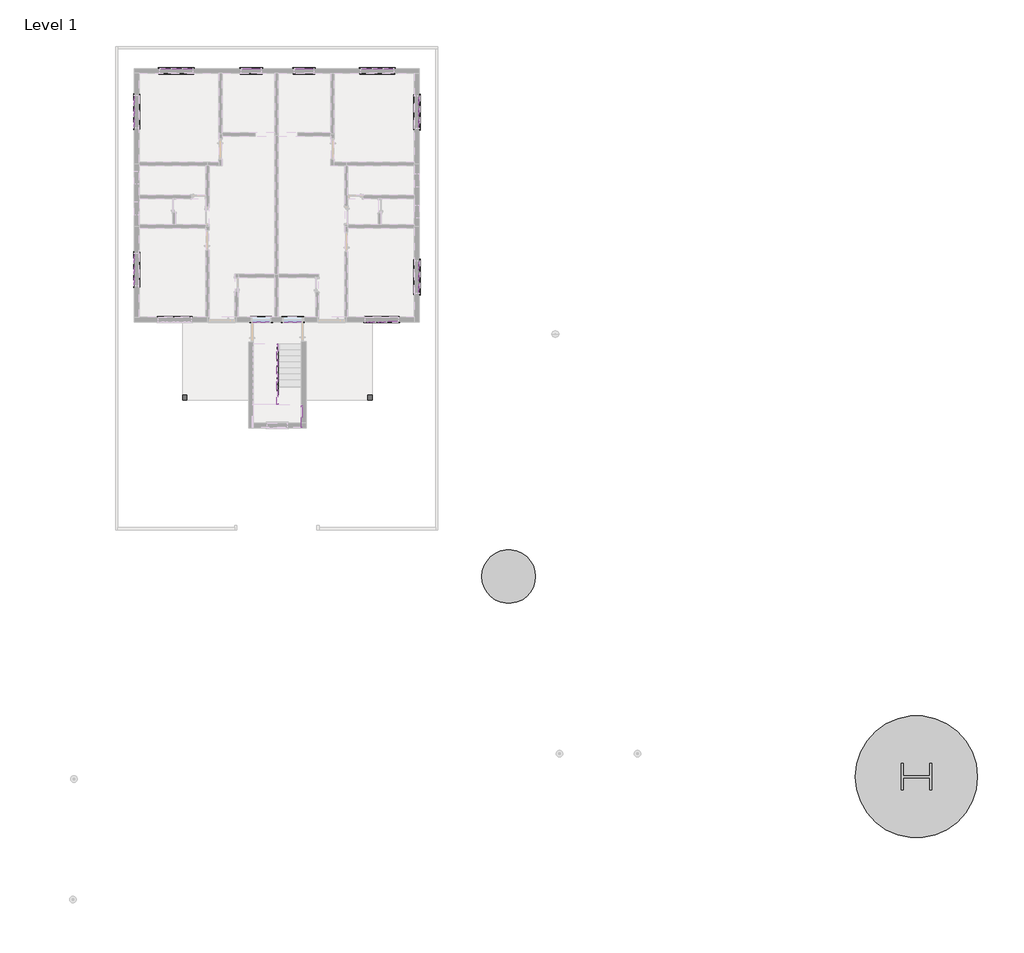
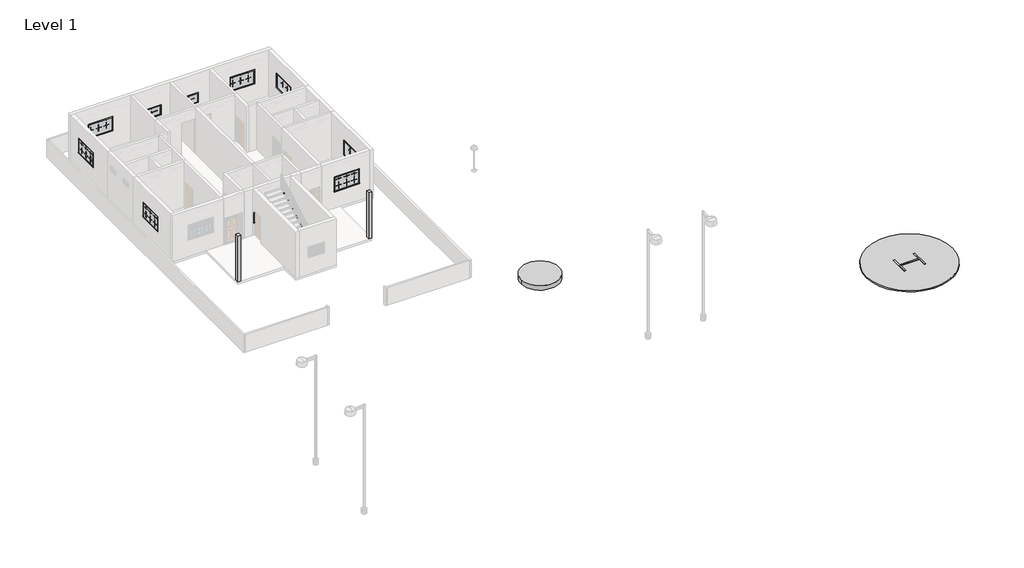
# One storey, part 4 of 4: 75 proxies, 5 members.
"""IFC4 building model written with IfcOpenShell, lengths in millimetres."""

from ifc_helpers import new_model, si_unit, frame, origin, place, context, project, spatial, polyline, outline, extrude, transform, mapped, element, save
from components import roads_7a27419f, generic_models_1_generic_models_1_f4687d58, m_muntin_pattern_2x2_m_muntin_pattern_2x2_be83c6ce, m_muntin_pattern_2x2_m_muntin_pattern_2x2_d2526705, m_muntin_pattern_2x2_m_muntin_pattern_2x2_b257745b, m_muntin_pattern_2x2_m_muntin_pattern_2x2_3c44882e, m_muntin_pattern_2x2_m_muntin_pattern_2x2_c118e93d, m_trim_window_exterior_flat_with_sill_30a8f3cc, m_trim_window_exterior_flat_with_sill_78b3ef69, m_trim_window_interior_flat_picture_frame_90bf1a90, m_trim_window_interior_flat_picture_frame_87bc748b

model = new_model("IFC4")

# Units and contexts
model_context = context("Model", 3, world=origin())
ifc_project = project(units=[si_unit("LENGTHUNIT", "METRE", prefix="MILLI")], contexts=[model_context])

# Site, building, storey
site = spatial("IfcSite", under=ifc_project)
building = spatial("IfcBuilding", under=site)
storey = spatial("IfcBuildingStorey", under=building, Name="Level 1", Elevation=0.0)

# Proxies
placement = place(None, origin())
roads_shape = roads_7a27419f(model_context)
element("IfcBuildingElementProxy", 1, Name="Roads", at=placement, inside=storey, context=model_context, shape_type="MappedRepresentation", body=[
    mapped(roads_shape, transform((0.0, 0.0, 0.0), x_axis=(1.0, 0.0, 0.0), y_axis=(0.0, 1.0, 0.0), z_axis=(0.0, 0.0, 1.0))),
])
generic_models_1_generic_models_1_shape = generic_models_1_generic_models_1_f4687d58(model_context)
element("IfcBuildingElementProxy", 2, Name="Generic Models 1 : Generic Models 1", ObjectType="Generic Models 1 : Generic Models 1", at=placement, inside=storey, context=model_context, shape_type="MappedRepresentation", body=[
    mapped(generic_models_1_generic_models_1_shape, transform((0.0, 0.0, 0.0), x_axis=(1.0, 0.0, 0.0), y_axis=(0.0, 1.0, 0.0), z_axis=(0.0, 0.0, 1.0))),
])
m_muntin_pattern_2x2_m_muntin_pattern_2x2_shape = m_muntin_pattern_2x2_m_muntin_pattern_2x2_be83c6ce(model_context)
element("IfcBuildingElementProxy", 3, Name="M_Muntin Pattern_2x2 : M_Muntin Pattern_2x2", ObjectType="M_Muntin Pattern_2x2 : M_Muntin Pattern_2x2", at=placement, inside=storey, context=model_context, shape_type="MappedRepresentation", body=[
    mapped(m_muntin_pattern_2x2_m_muntin_pattern_2x2_shape, transform((-12105.0132915, 19636.711641, 1289.05), x_axis=(1.0, 0.0, 0.0), y_axis=(0.0, 1.0, 0.0), z_axis=(0.0, 0.0, 1.0))),
])
element("IfcBuildingElementProxy", 4, Name="M_Muntin Pattern_2x2 : M_Muntin Pattern_2x2", ObjectType="M_Muntin Pattern_2x2 : M_Muntin Pattern_2x2", at=placement, inside=storey, context=model_context, shape_type="MappedRepresentation", body=[
    mapped(m_muntin_pattern_2x2_m_muntin_pattern_2x2_shape, transform((-13532.7049582, 17146.4533076, 1289.05), x_axis=(0.0, 1.0, 0.0), y_axis=(-1.0, 0.0, 0.0), z_axis=(0.0, 0.0, 1.0))),
])
element("IfcBuildingElementProxy", 5, Name="M_Muntin Pattern_2x2 : M_Muntin Pattern_2x2", ObjectType="M_Muntin Pattern_2x2 : M_Muntin Pattern_2x2", at=placement, inside=storey, context=model_context, shape_type="MappedRepresentation", body=[
    mapped(m_muntin_pattern_2x2_m_muntin_pattern_2x2_shape, transform((-2808.6132915, 19636.711641, 1289.05), x_axis=(1.0, 0.0, 0.0), y_axis=(0.0, 1.0, 0.0), z_axis=(0.0, 0.0, 1.0))),
])
element("IfcBuildingElementProxy", 6, Name="M_Muntin Pattern_2x2 : M_Muntin Pattern_2x2", ObjectType="M_Muntin Pattern_2x2 : M_Muntin Pattern_2x2", at=placement, inside=storey, context=model_context, shape_type="MappedRepresentation", body=[
    mapped(m_muntin_pattern_2x2_m_muntin_pattern_2x2_shape, transform((-369.1549582, 18132.8199743, 1289.05), x_axis=(0.0, -1.0, 0.0), y_axis=(1.0, 0.0, 0.0), z_axis=(0.0, 0.0, 1.0))),
])
element("IfcBuildingElementProxy", 7, Name="M_Muntin Pattern_2x2 : M_Muntin Pattern_2x2", ObjectType="M_Muntin Pattern_2x2 : M_Muntin Pattern_2x2", at=placement, inside=storey, context=model_context, shape_type="MappedRepresentation", body=[
    mapped(m_muntin_pattern_2x2_m_muntin_pattern_2x2_shape, transform((-369.1549582, 10487.4199743, 1289.05), x_axis=(0.0, -1.0, 0.0), y_axis=(1.0, 0.0, 0.0), z_axis=(0.0, 0.0, 1.0))),
])
element("IfcBuildingElementProxy", 8, Name="M_Muntin Pattern_2x2 : M_Muntin Pattern_2x2", ObjectType="M_Muntin Pattern_2x2 : M_Muntin Pattern_2x2", at=placement, inside=storey, context=model_context, shape_type="MappedRepresentation", body=[
    mapped(m_muntin_pattern_2x2_m_muntin_pattern_2x2_shape, transform((-1599.9966249, 7920.961641, 1289.05), x_axis=(-1.0, 0.0, 0.0), y_axis=(0.0, -1.0, 0.0), z_axis=(0.0, 0.0, 1.0))),
])
element("IfcBuildingElementProxy", 9, Name="M_Muntin Pattern_2x2 : M_Muntin Pattern_2x2", ObjectType="M_Muntin Pattern_2x2 : M_Muntin Pattern_2x2", at=placement, inside=storey, context=model_context, shape_type="MappedRepresentation", body=[
    mapped(m_muntin_pattern_2x2_m_muntin_pattern_2x2_shape, transform((-13532.7049582, 9834.4283076, 1289.05), x_axis=(0.0, 1.0, 0.0), y_axis=(-1.0, 0.0, 0.0), z_axis=(0.0, 0.0, 1.0))),
])
m_muntin_pattern_2x2_m_muntin_pattern_2x2_2_shape = m_muntin_pattern_2x2_m_muntin_pattern_2x2_d2526705(model_context)
element("IfcBuildingElementProxy", 10, Name="M_Muntin Pattern_2x2 : M_Muntin Pattern_2x2", ObjectType="M_Muntin Pattern_2x2 : M_Muntin Pattern_2x2", at=placement, inside=storey, context=model_context, shape_type="MappedRepresentation", body=[
    mapped(m_muntin_pattern_2x2_m_muntin_pattern_2x2_2_shape, transform((-11093.2466249, 19636.711641, 1289.05), x_axis=(-1.0, 0.0, 0.0), y_axis=(0.0, -1.0, 0.0), z_axis=(0.0, 0.0, 1.0))),
])
element("IfcBuildingElementProxy", 11, Name="M_Muntin Pattern_2x2 : M_Muntin Pattern_2x2", ObjectType="M_Muntin Pattern_2x2 : M_Muntin Pattern_2x2", at=placement, inside=storey, context=model_context, shape_type="MappedRepresentation", body=[
    mapped(m_muntin_pattern_2x2_m_muntin_pattern_2x2_2_shape, transform((-11599.1299582, 19636.711641, 1289.05), x_axis=(-1.0, 0.0, 0.0), y_axis=(0.0, -1.0, 0.0), z_axis=(0.0, 0.0, 1.0))),
])
element("IfcBuildingElementProxy", 12, Name="M_Muntin Pattern_2x2 : M_Muntin Pattern_2x2", ObjectType="M_Muntin Pattern_2x2 : M_Muntin Pattern_2x2", at=placement, inside=storey, context=model_context, shape_type="MappedRepresentation", body=[
    mapped(m_muntin_pattern_2x2_m_muntin_pattern_2x2_2_shape, transform((-13532.7049582, 18158.2199743, 1289.05), x_axis=(0.0, -1.0, 0.0), y_axis=(1.0, 0.0, 0.0), z_axis=(0.0, 0.0, 1.0))),
])
element("IfcBuildingElementProxy", 13, Name="M_Muntin Pattern_2x2 : M_Muntin Pattern_2x2", ObjectType="M_Muntin Pattern_2x2 : M_Muntin Pattern_2x2", at=placement, inside=storey, context=model_context, shape_type="MappedRepresentation", body=[
    mapped(m_muntin_pattern_2x2_m_muntin_pattern_2x2_2_shape, transform((-13532.7049582, 17652.336641, 1289.05), x_axis=(0.0, -1.0, 0.0), y_axis=(1.0, 0.0, 0.0), z_axis=(0.0, 0.0, 1.0))),
])
element("IfcBuildingElementProxy", 14, Name="M_Muntin Pattern_2x2 : M_Muntin Pattern_2x2", ObjectType="M_Muntin Pattern_2x2 : M_Muntin Pattern_2x2", at=placement, inside=storey, context=model_context, shape_type="MappedRepresentation", body=[
    mapped(m_muntin_pattern_2x2_m_muntin_pattern_2x2_2_shape, transform((-1796.8466249, 19636.711641, 1289.05), x_axis=(-1.0, 0.0, 0.0), y_axis=(0.0, -1.0, 0.0), z_axis=(0.0, 0.0, 1.0))),
])
element("IfcBuildingElementProxy", 15, Name="M_Muntin Pattern_2x2 : M_Muntin Pattern_2x2", ObjectType="M_Muntin Pattern_2x2 : M_Muntin Pattern_2x2", at=placement, inside=storey, context=model_context, shape_type="MappedRepresentation", body=[
    mapped(m_muntin_pattern_2x2_m_muntin_pattern_2x2_2_shape, transform((-2302.7299582, 19636.711641, 1289.05), x_axis=(-1.0, 0.0, 0.0), y_axis=(0.0, -1.0, 0.0), z_axis=(0.0, 0.0, 1.0))),
])
element("IfcBuildingElementProxy", 16, Name="M_Muntin Pattern_2x2 : M_Muntin Pattern_2x2", ObjectType="M_Muntin Pattern_2x2 : M_Muntin Pattern_2x2", at=placement, inside=storey, context=model_context, shape_type="MappedRepresentation", body=[
    mapped(m_muntin_pattern_2x2_m_muntin_pattern_2x2_2_shape, transform((-369.1549582, 17121.0533076, 1289.05), x_axis=(0.0, 1.0, 0.0), y_axis=(-1.0, 0.0, 0.0), z_axis=(0.0, 0.0, 1.0))),
])
element("IfcBuildingElementProxy", 17, Name="M_Muntin Pattern_2x2 : M_Muntin Pattern_2x2", ObjectType="M_Muntin Pattern_2x2 : M_Muntin Pattern_2x2", at=placement, inside=storey, context=model_context, shape_type="MappedRepresentation", body=[
    mapped(m_muntin_pattern_2x2_m_muntin_pattern_2x2_2_shape, transform((-369.1549582, 17626.936641, 1289.05), x_axis=(0.0, 1.0, 0.0), y_axis=(-1.0, 0.0, 0.0), z_axis=(0.0, 0.0, 1.0))),
])
element("IfcBuildingElementProxy", 18, Name="M_Muntin Pattern_2x2 : M_Muntin Pattern_2x2", ObjectType="M_Muntin Pattern_2x2 : M_Muntin Pattern_2x2", at=placement, inside=storey, context=model_context, shape_type="MappedRepresentation", body=[
    mapped(m_muntin_pattern_2x2_m_muntin_pattern_2x2_2_shape, transform((-369.1549582, 9475.6533076, 1289.05), x_axis=(0.0, 1.0, 0.0), y_axis=(-1.0, 0.0, 0.0), z_axis=(0.0, 0.0, 1.0))),
])
element("IfcBuildingElementProxy", 19, Name="M_Muntin Pattern_2x2 : M_Muntin Pattern_2x2", ObjectType="M_Muntin Pattern_2x2 : M_Muntin Pattern_2x2", at=placement, inside=storey, context=model_context, shape_type="MappedRepresentation", body=[
    mapped(m_muntin_pattern_2x2_m_muntin_pattern_2x2_2_shape, transform((-369.1549582, 9981.536641, 1289.05), x_axis=(0.0, 1.0, 0.0), y_axis=(-1.0, 0.0, 0.0), z_axis=(0.0, 0.0, 1.0))),
])
element("IfcBuildingElementProxy", 20, Name="M_Muntin Pattern_2x2 : M_Muntin Pattern_2x2", ObjectType="M_Muntin Pattern_2x2 : M_Muntin Pattern_2x2", at=placement, inside=storey, context=model_context, shape_type="MappedRepresentation", body=[
    mapped(m_muntin_pattern_2x2_m_muntin_pattern_2x2_2_shape, transform((-2611.7632915, 7920.961641, 1289.05), x_axis=(1.0, 0.0, 0.0), y_axis=(0.0, 1.0, 0.0), z_axis=(0.0, 0.0, 1.0))),
])
element("IfcBuildingElementProxy", 21, Name="M_Muntin Pattern_2x2 : M_Muntin Pattern_2x2", ObjectType="M_Muntin Pattern_2x2 : M_Muntin Pattern_2x2", at=placement, inside=storey, context=model_context, shape_type="MappedRepresentation", body=[
    mapped(m_muntin_pattern_2x2_m_muntin_pattern_2x2_2_shape, transform((-2105.8799582, 7920.961641, 1289.05), x_axis=(1.0, 0.0, 0.0), y_axis=(0.0, 1.0, 0.0), z_axis=(0.0, 0.0, 1.0))),
])
element("IfcBuildingElementProxy", 22, Name="M_Muntin Pattern_2x2 : M_Muntin Pattern_2x2", ObjectType="M_Muntin Pattern_2x2 : M_Muntin Pattern_2x2", at=placement, inside=storey, context=model_context, shape_type="MappedRepresentation", body=[
    mapped(m_muntin_pattern_2x2_m_muntin_pattern_2x2_2_shape, transform((-13532.7049582, 10846.1949743, 1289.05), x_axis=(0.0, -1.0, 0.0), y_axis=(1.0, 0.0, 0.0), z_axis=(0.0, 0.0, 1.0))),
])
element("IfcBuildingElementProxy", 23, Name="M_Muntin Pattern_2x2 : M_Muntin Pattern_2x2", ObjectType="M_Muntin Pattern_2x2 : M_Muntin Pattern_2x2", at=placement, inside=storey, context=model_context, shape_type="MappedRepresentation", body=[
    mapped(m_muntin_pattern_2x2_m_muntin_pattern_2x2_2_shape, transform((-13532.7049582, 10340.311641, 1289.05), x_axis=(0.0, -1.0, 0.0), y_axis=(1.0, 0.0, 0.0), z_axis=(0.0, 0.0, 1.0))),
])
m_muntin_pattern_2x2_m_muntin_pattern_2x2_3_shape = m_muntin_pattern_2x2_m_muntin_pattern_2x2_b257745b(model_context)
element("IfcBuildingElementProxy", 24, Name="M_Muntin Pattern_2x2 : M_Muntin Pattern_2x2", ObjectType="M_Muntin Pattern_2x2 : M_Muntin Pattern_2x2", at=placement, inside=storey, context=model_context, shape_type="MappedRepresentation", body=[
    mapped(m_muntin_pattern_2x2_m_muntin_pattern_2x2_3_shape, transform((-11599.1299582, 19636.711641, 1889.05), x_axis=(1.0, 0.0, 0.0), y_axis=(0.0, 1.0, 0.0), z_axis=(0.0, 0.0, 1.0))),
])
element("IfcBuildingElementProxy", 25, Name="M_Muntin Pattern_2x2 : M_Muntin Pattern_2x2", ObjectType="M_Muntin Pattern_2x2 : M_Muntin Pattern_2x2", at=placement, inside=storey, context=model_context, shape_type="MappedRepresentation", body=[
    mapped(m_muntin_pattern_2x2_m_muntin_pattern_2x2_3_shape, transform((-11093.2466249, 19636.711641, 1889.05), x_axis=(1.0, 0.0, 0.0), y_axis=(0.0, 1.0, 0.0), z_axis=(0.0, 0.0, 1.0))),
])
element("IfcBuildingElementProxy", 26, Name="M_Muntin Pattern_2x2 : M_Muntin Pattern_2x2", ObjectType="M_Muntin Pattern_2x2 : M_Muntin Pattern_2x2", at=placement, inside=storey, context=model_context, shape_type="MappedRepresentation", body=[
    mapped(m_muntin_pattern_2x2_m_muntin_pattern_2x2_3_shape, transform((-12105.0132915, 19636.711641, 1889.05), x_axis=(1.0, 0.0, 0.0), y_axis=(0.0, 1.0, 0.0), z_axis=(0.0, 0.0, 1.0))),
])
element("IfcBuildingElementProxy", 27, Name="M_Muntin Pattern_2x2 : M_Muntin Pattern_2x2", ObjectType="M_Muntin Pattern_2x2 : M_Muntin Pattern_2x2", at=placement, inside=storey, context=model_context, shape_type="MappedRepresentation", body=[
    mapped(m_muntin_pattern_2x2_m_muntin_pattern_2x2_3_shape, transform((-13532.7049582, 17652.336641, 1889.05), x_axis=(0.0, 1.0, 0.0), y_axis=(-1.0, 0.0, 0.0), z_axis=(0.0, 0.0, 1.0))),
])
element("IfcBuildingElementProxy", 28, Name="M_Muntin Pattern_2x2 : M_Muntin Pattern_2x2", ObjectType="M_Muntin Pattern_2x2 : M_Muntin Pattern_2x2", at=placement, inside=storey, context=model_context, shape_type="MappedRepresentation", body=[
    mapped(m_muntin_pattern_2x2_m_muntin_pattern_2x2_3_shape, transform((-13532.7049582, 18158.2199743, 1889.05), x_axis=(0.0, 1.0, 0.0), y_axis=(-1.0, 0.0, 0.0), z_axis=(0.0, 0.0, 1.0))),
])
element("IfcBuildingElementProxy", 29, Name="M_Muntin Pattern_2x2 : M_Muntin Pattern_2x2", ObjectType="M_Muntin Pattern_2x2 : M_Muntin Pattern_2x2", at=placement, inside=storey, context=model_context, shape_type="MappedRepresentation", body=[
    mapped(m_muntin_pattern_2x2_m_muntin_pattern_2x2_3_shape, transform((-13532.7049582, 17146.4533076, 1889.05), x_axis=(0.0, 1.0, 0.0), y_axis=(-1.0, 0.0, 0.0), z_axis=(0.0, 0.0, 1.0))),
])
element("IfcBuildingElementProxy", 30, Name="M_Muntin Pattern_2x2 : M_Muntin Pattern_2x2", ObjectType="M_Muntin Pattern_2x2 : M_Muntin Pattern_2x2", at=placement, inside=storey, context=model_context, shape_type="MappedRepresentation", body=[
    mapped(m_muntin_pattern_2x2_m_muntin_pattern_2x2_3_shape, transform((-2302.7299582, 19636.711641, 1889.05), x_axis=(1.0, 0.0, 0.0), y_axis=(0.0, 1.0, 0.0), z_axis=(0.0, 0.0, 1.0))),
])
element("IfcBuildingElementProxy", 31, Name="M_Muntin Pattern_2x2 : M_Muntin Pattern_2x2", ObjectType="M_Muntin Pattern_2x2 : M_Muntin Pattern_2x2", at=placement, inside=storey, context=model_context, shape_type="MappedRepresentation", body=[
    mapped(m_muntin_pattern_2x2_m_muntin_pattern_2x2_3_shape, transform((-1796.8466249, 19636.711641, 1889.05), x_axis=(1.0, 0.0, 0.0), y_axis=(0.0, 1.0, 0.0), z_axis=(0.0, 0.0, 1.0))),
])
element("IfcBuildingElementProxy", 32, Name="M_Muntin Pattern_2x2 : M_Muntin Pattern_2x2", ObjectType="M_Muntin Pattern_2x2 : M_Muntin Pattern_2x2", at=placement, inside=storey, context=model_context, shape_type="MappedRepresentation", body=[
    mapped(m_muntin_pattern_2x2_m_muntin_pattern_2x2_3_shape, transform((-2808.6132915, 19636.711641, 1889.05), x_axis=(1.0, 0.0, 0.0), y_axis=(0.0, 1.0, 0.0), z_axis=(0.0, 0.0, 1.0))),
])
element("IfcBuildingElementProxy", 33, Name="M_Muntin Pattern_2x2 : M_Muntin Pattern_2x2", ObjectType="M_Muntin Pattern_2x2 : M_Muntin Pattern_2x2", at=placement, inside=storey, context=model_context, shape_type="MappedRepresentation", body=[
    mapped(m_muntin_pattern_2x2_m_muntin_pattern_2x2_3_shape, transform((-369.1549582, 17626.936641, 1889.05), x_axis=(0.0, -1.0, 0.0), y_axis=(1.0, 0.0, 0.0), z_axis=(0.0, 0.0, 1.0))),
])
element("IfcBuildingElementProxy", 34, Name="M_Muntin Pattern_2x2 : M_Muntin Pattern_2x2", ObjectType="M_Muntin Pattern_2x2 : M_Muntin Pattern_2x2", at=placement, inside=storey, context=model_context, shape_type="MappedRepresentation", body=[
    mapped(m_muntin_pattern_2x2_m_muntin_pattern_2x2_3_shape, transform((-369.1549582, 17121.0533076, 1889.05), x_axis=(0.0, -1.0, 0.0), y_axis=(1.0, 0.0, 0.0), z_axis=(0.0, 0.0, 1.0))),
])
element("IfcBuildingElementProxy", 35, Name="M_Muntin Pattern_2x2 : M_Muntin Pattern_2x2", ObjectType="M_Muntin Pattern_2x2 : M_Muntin Pattern_2x2", at=placement, inside=storey, context=model_context, shape_type="MappedRepresentation", body=[
    mapped(m_muntin_pattern_2x2_m_muntin_pattern_2x2_3_shape, transform((-369.1549582, 18132.8199743, 1889.05), x_axis=(0.0, -1.0, 0.0), y_axis=(1.0, 0.0, 0.0), z_axis=(0.0, 0.0, 1.0))),
])
element("IfcBuildingElementProxy", 36, Name="M_Muntin Pattern_2x2 : M_Muntin Pattern_2x2", ObjectType="M_Muntin Pattern_2x2 : M_Muntin Pattern_2x2", at=placement, inside=storey, context=model_context, shape_type="MappedRepresentation", body=[
    mapped(m_muntin_pattern_2x2_m_muntin_pattern_2x2_3_shape, transform((-369.1549582, 9981.536641, 1889.05), x_axis=(0.0, -1.0, 0.0), y_axis=(1.0, 0.0, 0.0), z_axis=(0.0, 0.0, 1.0))),
])
element("IfcBuildingElementProxy", 37, Name="M_Muntin Pattern_2x2 : M_Muntin Pattern_2x2", ObjectType="M_Muntin Pattern_2x2 : M_Muntin Pattern_2x2", at=placement, inside=storey, context=model_context, shape_type="MappedRepresentation", body=[
    mapped(m_muntin_pattern_2x2_m_muntin_pattern_2x2_3_shape, transform((-369.1549582, 9475.6533076, 1889.05), x_axis=(0.0, -1.0, 0.0), y_axis=(1.0, 0.0, 0.0), z_axis=(0.0, 0.0, 1.0))),
])
element("IfcBuildingElementProxy", 38, Name="M_Muntin Pattern_2x2 : M_Muntin Pattern_2x2", ObjectType="M_Muntin Pattern_2x2 : M_Muntin Pattern_2x2", at=placement, inside=storey, context=model_context, shape_type="MappedRepresentation", body=[
    mapped(m_muntin_pattern_2x2_m_muntin_pattern_2x2_3_shape, transform((-369.1549582, 10487.4199743, 1889.05), x_axis=(0.0, -1.0, 0.0), y_axis=(1.0, 0.0, 0.0), z_axis=(0.0, 0.0, 1.0))),
])
element("IfcBuildingElementProxy", 39, Name="M_Muntin Pattern_2x2 : M_Muntin Pattern_2x2", ObjectType="M_Muntin Pattern_2x2 : M_Muntin Pattern_2x2", at=placement, inside=storey, context=model_context, shape_type="MappedRepresentation", body=[
    mapped(m_muntin_pattern_2x2_m_muntin_pattern_2x2_3_shape, transform((-2105.8799582, 7920.961641, 1889.05), x_axis=(-1.0, 0.0, 0.0), y_axis=(0.0, -1.0, 0.0), z_axis=(0.0, 0.0, 1.0))),
])
element("IfcBuildingElementProxy", 40, Name="M_Muntin Pattern_2x2 : M_Muntin Pattern_2x2", ObjectType="M_Muntin Pattern_2x2 : M_Muntin Pattern_2x2", at=placement, inside=storey, context=model_context, shape_type="MappedRepresentation", body=[
    mapped(m_muntin_pattern_2x2_m_muntin_pattern_2x2_3_shape, transform((-2611.7632915, 7920.961641, 1889.05), x_axis=(-1.0, 0.0, 0.0), y_axis=(0.0, -1.0, 0.0), z_axis=(0.0, 0.0, 1.0))),
])
element("IfcBuildingElementProxy", 41, Name="M_Muntin Pattern_2x2 : M_Muntin Pattern_2x2", ObjectType="M_Muntin Pattern_2x2 : M_Muntin Pattern_2x2", at=placement, inside=storey, context=model_context, shape_type="MappedRepresentation", body=[
    mapped(m_muntin_pattern_2x2_m_muntin_pattern_2x2_3_shape, transform((-1599.9966249, 7920.961641, 1889.05), x_axis=(-1.0, 0.0, 0.0), y_axis=(0.0, -1.0, 0.0), z_axis=(0.0, 0.0, 1.0))),
])
element("IfcBuildingElementProxy", 42, Name="M_Muntin Pattern_2x2 : M_Muntin Pattern_2x2", ObjectType="M_Muntin Pattern_2x2 : M_Muntin Pattern_2x2", at=placement, inside=storey, context=model_context, shape_type="MappedRepresentation", body=[
    mapped(m_muntin_pattern_2x2_m_muntin_pattern_2x2_3_shape, transform((-13532.7049582, 10340.311641, 1889.05), x_axis=(0.0, 1.0, 0.0), y_axis=(-1.0, 0.0, 0.0), z_axis=(0.0, 0.0, 1.0))),
])
element("IfcBuildingElementProxy", 43, Name="M_Muntin Pattern_2x2 : M_Muntin Pattern_2x2", ObjectType="M_Muntin Pattern_2x2 : M_Muntin Pattern_2x2", at=placement, inside=storey, context=model_context, shape_type="MappedRepresentation", body=[
    mapped(m_muntin_pattern_2x2_m_muntin_pattern_2x2_3_shape, transform((-13532.7049582, 10846.1949743, 1889.05), x_axis=(0.0, 1.0, 0.0), y_axis=(-1.0, 0.0, 0.0), z_axis=(0.0, 0.0, 1.0))),
])
element("IfcBuildingElementProxy", 44, Name="M_Muntin Pattern_2x2 : M_Muntin Pattern_2x2", ObjectType="M_Muntin Pattern_2x2 : M_Muntin Pattern_2x2", at=placement, inside=storey, context=model_context, shape_type="MappedRepresentation", body=[
    mapped(m_muntin_pattern_2x2_m_muntin_pattern_2x2_3_shape, transform((-13532.7049582, 9834.4283076, 1889.05), x_axis=(0.0, 1.0, 0.0), y_axis=(-1.0, 0.0, 0.0), z_axis=(0.0, 0.0, 1.0))),
])
m_muntin_pattern_2x2_m_muntin_pattern_2x2_4_shape = m_muntin_pattern_2x2_m_muntin_pattern_2x2_3c44882e(model_context)
element("IfcBuildingElementProxy", 45, Name="M_Muntin Pattern_2x2 : M_Muntin Pattern_2x2", ObjectType="M_Muntin Pattern_2x2 : M_Muntin Pattern_2x2", at=placement, inside=storey, context=model_context, shape_type="MappedRepresentation", body=[
    mapped(m_muntin_pattern_2x2_m_muntin_pattern_2x2_4_shape, transform((-8132.0299582, 19636.711641, 1589.05), x_axis=(1.0, 0.0, 0.0), y_axis=(0.0, 1.0, 0.0), z_axis=(0.0, 0.0, 1.0))),
])
element("IfcBuildingElementProxy", 46, Name="M_Muntin Pattern_2x2 : M_Muntin Pattern_2x2", ObjectType="M_Muntin Pattern_2x2 : M_Muntin Pattern_2x2", at=placement, inside=storey, context=model_context, shape_type="MappedRepresentation", body=[
    mapped(m_muntin_pattern_2x2_m_muntin_pattern_2x2_4_shape, transform((-5693.6299582, 19636.711641, 1589.05), x_axis=(1.0, 0.0, 0.0), y_axis=(0.0, 1.0, 0.0), z_axis=(0.0, 0.0, 1.0))),
])
element("IfcBuildingElementProxy", 47, Name="M_Muntin Pattern_2x2 : M_Muntin Pattern_2x2", ObjectType="M_Muntin Pattern_2x2 : M_Muntin Pattern_2x2", at=placement, inside=storey, context=model_context, shape_type="MappedRepresentation", body=[
    mapped(m_muntin_pattern_2x2_m_muntin_pattern_2x2_4_shape, transform((-7680.5269054, 7920.961641, 1269.85), x_axis=(-1.0, 0.0, 0.0), y_axis=(0.0, -1.0, 0.0), z_axis=(0.0, 0.0, 1.0))),
])
element("IfcBuildingElementProxy", 48, Name="M_Muntin Pattern_2x2 : M_Muntin Pattern_2x2", ObjectType="M_Muntin Pattern_2x2 : M_Muntin Pattern_2x2", at=placement, inside=storey, context=model_context, shape_type="MappedRepresentation", body=[
    mapped(m_muntin_pattern_2x2_m_muntin_pattern_2x2_4_shape, transform((-6219.2331554, 7920.961641, 1269.85), x_axis=(-1.0, 0.0, 0.0), y_axis=(0.0, -1.0, 0.0), z_axis=(0.0, 0.0, 1.0))),
])
m_muntin_pattern_2x2_m_muntin_pattern_2x2_5_shape = m_muntin_pattern_2x2_m_muntin_pattern_2x2_c118e93d(model_context)
element("IfcBuildingElementProxy", 49, Name="M_Muntin Pattern_2x2 : M_Muntin Pattern_2x2", ObjectType="M_Muntin Pattern_2x2 : M_Muntin Pattern_2x2", at=placement, inside=storey, context=model_context, shape_type="MappedRepresentation", body=[
    mapped(m_muntin_pattern_2x2_m_muntin_pattern_2x2_5_shape, transform((-8132.0299582, 19636.711641, 1289.05), x_axis=(1.0, 0.0, 0.0), y_axis=(0.0, 1.0, 0.0), z_axis=(0.0, 0.0, 1.0))),
])
element("IfcBuildingElementProxy", 50, Name="M_Muntin Pattern_2x2 : M_Muntin Pattern_2x2", ObjectType="M_Muntin Pattern_2x2 : M_Muntin Pattern_2x2", at=placement, inside=storey, context=model_context, shape_type="MappedRepresentation", body=[
    mapped(m_muntin_pattern_2x2_m_muntin_pattern_2x2_5_shape, transform((-5693.6299582, 19636.711641, 1289.05), x_axis=(1.0, 0.0, 0.0), y_axis=(0.0, 1.0, 0.0), z_axis=(0.0, 0.0, 1.0))),
])
element("IfcBuildingElementProxy", 51, Name="M_Muntin Pattern_2x2 : M_Muntin Pattern_2x2", ObjectType="M_Muntin Pattern_2x2 : M_Muntin Pattern_2x2", at=placement, inside=storey, context=model_context, shape_type="MappedRepresentation", body=[
    mapped(m_muntin_pattern_2x2_m_muntin_pattern_2x2_5_shape, transform((-7680.5269054, 7920.961641, 969.85), x_axis=(-1.0, 0.0, 0.0), y_axis=(0.0, -1.0, 0.0), z_axis=(0.0, 0.0, 1.0))),
])
element("IfcBuildingElementProxy", 52, Name="M_Muntin Pattern_2x2 : M_Muntin Pattern_2x2", ObjectType="M_Muntin Pattern_2x2 : M_Muntin Pattern_2x2", at=placement, inside=storey, context=model_context, shape_type="MappedRepresentation", body=[
    mapped(m_muntin_pattern_2x2_m_muntin_pattern_2x2_5_shape, transform((-6219.2331554, 7920.961641, 969.85), x_axis=(-1.0, 0.0, 0.0), y_axis=(0.0, -1.0, 0.0), z_axis=(0.0, 0.0, 1.0))),
])
m_trim_window_exterior_flat_with_sill_shape = m_trim_window_exterior_flat_with_sill_30a8f3cc(model_context)
element("IfcBuildingElementProxy", 53, Name="M_Trim-Window-Exterior-Flat : with Sill", ObjectType="M_Trim-Window-Exterior-Flat : with Sill", at=placement, inside=storey, context=model_context, shape_type="MappedRepresentation", body=[
    mapped(m_trim_window_exterior_flat_with_sill_shape, transform((-11599.1299582, 19646.236641, 2119.2), x_axis=(-1.0, 0.0, 0.0), y_axis=(0.0, 0.0, 1.0), z_axis=(0.0, 1.0, 0.0))),
])
element("IfcBuildingElementProxy", 54, Name="M_Trim-Window-Exterior-Flat : with Sill", ObjectType="M_Trim-Window-Exterior-Flat : with Sill", at=placement, inside=storey, context=model_context, shape_type="MappedRepresentation", body=[
    mapped(m_trim_window_exterior_flat_with_sill_shape, transform((-13542.2299582, 17652.336641, 2119.2), x_axis=(0.0, -1.0, 0.0), y_axis=(0.0, 0.0, 1.0), z_axis=(-1.0, 0.0, 0.0))),
])
element("IfcBuildingElementProxy", 55, Name="M_Trim-Window-Exterior-Flat : with Sill", ObjectType="M_Trim-Window-Exterior-Flat : with Sill", at=placement, inside=storey, context=model_context, shape_type="MappedRepresentation", body=[
    mapped(m_trim_window_exterior_flat_with_sill_shape, transform((-2302.7299582, 19646.236641, 2119.2), x_axis=(-1.0, 0.0, 0.0), y_axis=(0.0, 0.0, 1.0), z_axis=(0.0, 1.0, 0.0))),
])
element("IfcBuildingElementProxy", 56, Name="M_Trim-Window-Exterior-Flat : with Sill", ObjectType="M_Trim-Window-Exterior-Flat : with Sill", at=placement, inside=storey, context=model_context, shape_type="MappedRepresentation", body=[
    mapped(m_trim_window_exterior_flat_with_sill_shape, transform((-359.6299582, 17626.936641, 2119.2), x_axis=(0.0, 1.0, 0.0), y_axis=(0.0, 0.0, 1.0), z_axis=(1.0, 0.0, 0.0))),
])
element("IfcBuildingElementProxy", 57, Name="M_Trim-Window-Exterior-Flat : with Sill", ObjectType="M_Trim-Window-Exterior-Flat : with Sill", at=placement, inside=storey, context=model_context, shape_type="MappedRepresentation", body=[
    mapped(m_trim_window_exterior_flat_with_sill_shape, transform((-359.6299582, 9981.536641, 2119.2), x_axis=(0.0, 1.0, 0.0), y_axis=(0.0, 0.0, 1.0), z_axis=(1.0, 0.0, 0.0))),
])
element("IfcBuildingElementProxy", 58, Name="M_Trim-Window-Exterior-Flat : with Sill", ObjectType="M_Trim-Window-Exterior-Flat : with Sill", at=placement, inside=storey, context=model_context, shape_type="MappedRepresentation", body=[
    mapped(m_trim_window_exterior_flat_with_sill_shape, transform((-2105.8799582, 7911.436641, 2119.2), x_axis=(1.0, 0.0, 0.0), y_axis=(0.0, 0.0, 1.0), z_axis=(0.0, -1.0, 0.0))),
])
element("IfcBuildingElementProxy", 59, Name="M_Trim-Window-Exterior-Flat : with Sill", ObjectType="M_Trim-Window-Exterior-Flat : with Sill", at=placement, inside=storey, context=model_context, shape_type="MappedRepresentation", body=[
    mapped(m_trim_window_exterior_flat_with_sill_shape, transform((-13542.2299582, 10340.311641, 2119.2), x_axis=(0.0, -1.0, 0.0), y_axis=(0.0, 0.0, 1.0), z_axis=(-1.0, 0.0, 0.0))),
])
m_trim_window_exterior_flat_with_sill_2_shape = m_trim_window_exterior_flat_with_sill_78b3ef69(model_context)
element("IfcBuildingElementProxy", 60, Name="M_Trim-Window-Exterior-Flat : with Sill", ObjectType="M_Trim-Window-Exterior-Flat : with Sill", at=placement, inside=storey, context=model_context, shape_type="MappedRepresentation", body=[
    mapped(m_trim_window_exterior_flat_with_sill_2_shape, transform((-8132.0299582, 19646.236641, 1819.2), x_axis=(-1.0, 0.0, 0.0), y_axis=(0.0, 0.0, 1.0), z_axis=(0.0, 1.0, 0.0))),
])
element("IfcBuildingElementProxy", 61, Name="M_Trim-Window-Exterior-Flat : with Sill", ObjectType="M_Trim-Window-Exterior-Flat : with Sill", at=placement, inside=storey, context=model_context, shape_type="MappedRepresentation", body=[
    mapped(m_trim_window_exterior_flat_with_sill_2_shape, transform((-5693.6299582, 19646.236641, 1819.2), x_axis=(-1.0, 0.0, 0.0), y_axis=(0.0, 0.0, 1.0), z_axis=(0.0, 1.0, 0.0))),
])
element("IfcBuildingElementProxy", 62, Name="M_Trim-Window-Exterior-Flat : with Sill", ObjectType="M_Trim-Window-Exterior-Flat : with Sill", at=placement, inside=storey, context=model_context, shape_type="MappedRepresentation", body=[
    mapped(m_trim_window_exterior_flat_with_sill_2_shape, transform((-7680.5269054, 7911.436641, 1500.0), x_axis=(1.0, 0.0, 0.0), y_axis=(0.0, 0.0, 1.0), z_axis=(0.0, -1.0, 0.0))),
])
element("IfcBuildingElementProxy", 63, Name="M_Trim-Window-Exterior-Flat : with Sill", ObjectType="M_Trim-Window-Exterior-Flat : with Sill", at=placement, inside=storey, context=model_context, shape_type="MappedRepresentation", body=[
    mapped(m_trim_window_exterior_flat_with_sill_2_shape, transform((-6219.2331554, 7911.436641, 1500.0), x_axis=(1.0, 0.0, 0.0), y_axis=(0.0, 0.0, 1.0), z_axis=(0.0, -1.0, 0.0))),
])
m_trim_window_interior_flat_picture_frame_shape = m_trim_window_interior_flat_picture_frame_90bf1a90(model_context)
element("IfcBuildingElementProxy", 64, Name="M_Trim-Window-Interior-Flat : Picture Frame", ObjectType="M_Trim-Window-Interior-Flat : Picture Frame", at=placement, inside=storey, context=model_context, shape_type="MappedRepresentation", body=[
    mapped(m_trim_window_interior_flat_picture_frame_shape, transform((-11599.1299582, 19417.636641, 2119.2), x_axis=(1.0, 0.0, 0.0), y_axis=(0.0, 0.0, 1.0), z_axis=(0.0, -1.0, 0.0))),
])
element("IfcBuildingElementProxy", 65, Name="M_Trim-Window-Interior-Flat : Picture Frame", ObjectType="M_Trim-Window-Interior-Flat : Picture Frame", at=placement, inside=storey, context=model_context, shape_type="MappedRepresentation", body=[
    mapped(m_trim_window_interior_flat_picture_frame_shape, transform((-13313.6299582, 17652.336641, 2119.2), x_axis=(0.0, 1.0, 0.0), y_axis=(0.0, 0.0, 1.0), z_axis=(1.0, 0.0, 0.0))),
])
element("IfcBuildingElementProxy", 66, Name="M_Trim-Window-Interior-Flat : Picture Frame", ObjectType="M_Trim-Window-Interior-Flat : Picture Frame", at=placement, inside=storey, context=model_context, shape_type="MappedRepresentation", body=[
    mapped(m_trim_window_interior_flat_picture_frame_shape, transform((-2302.7299582, 19417.636641, 2119.2), x_axis=(1.0, 0.0, 0.0), y_axis=(0.0, 0.0, 1.0), z_axis=(0.0, -1.0, 0.0))),
])
element("IfcBuildingElementProxy", 67, Name="M_Trim-Window-Interior-Flat : Picture Frame", ObjectType="M_Trim-Window-Interior-Flat : Picture Frame", at=placement, inside=storey, context=model_context, shape_type="MappedRepresentation", body=[
    mapped(m_trim_window_interior_flat_picture_frame_shape, transform((-588.2299582, 17626.936641, 2119.2), x_axis=(0.0, -1.0, 0.0), y_axis=(0.0, 0.0, 1.0), z_axis=(-1.0, 0.0, 0.0))),
])
element("IfcBuildingElementProxy", 68, Name="M_Trim-Window-Interior-Flat : Picture Frame", ObjectType="M_Trim-Window-Interior-Flat : Picture Frame", at=placement, inside=storey, context=model_context, shape_type="MappedRepresentation", body=[
    mapped(m_trim_window_interior_flat_picture_frame_shape, transform((-588.2299582, 9981.536641, 2119.2), x_axis=(0.0, -1.0, 0.0), y_axis=(0.0, 0.0, 1.0), z_axis=(-1.0, 0.0, 0.0))),
])
element("IfcBuildingElementProxy", 69, Name="M_Trim-Window-Interior-Flat : Picture Frame", ObjectType="M_Trim-Window-Interior-Flat : Picture Frame", at=placement, inside=storey, context=model_context, shape_type="MappedRepresentation", body=[
    mapped(m_trim_window_interior_flat_picture_frame_shape, transform((-2105.8799582, 8140.036641, 2119.2), x_axis=(-1.0, 0.0, 0.0), y_axis=(0.0, 0.0, 1.0), z_axis=(0.0, 1.0, 0.0))),
])
element("IfcBuildingElementProxy", 70, Name="M_Trim-Window-Interior-Flat : Picture Frame", ObjectType="M_Trim-Window-Interior-Flat : Picture Frame", at=placement, inside=storey, context=model_context, shape_type="MappedRepresentation", body=[
    mapped(m_trim_window_interior_flat_picture_frame_shape, transform((-11668.9799582, 8140.036641, 2119.2), x_axis=(-1.0, 0.0, 0.0), y_axis=(0.0, 0.0, 1.0), z_axis=(0.0, 1.0, 0.0))),
])
element("IfcBuildingElementProxy", 71, Name="M_Trim-Window-Interior-Flat : Picture Frame", ObjectType="M_Trim-Window-Interior-Flat : Picture Frame", at=placement, inside=storey, context=model_context, shape_type="MappedRepresentation", body=[
    mapped(m_trim_window_interior_flat_picture_frame_shape, transform((-13313.6299582, 10340.311641, 2119.2), x_axis=(0.0, 1.0, 0.0), y_axis=(0.0, 0.0, 1.0), z_axis=(1.0, 0.0, 0.0))),
])
m_trim_window_interior_flat_picture_frame_2_shape = m_trim_window_interior_flat_picture_frame_87bc748b(model_context)
element("IfcBuildingElementProxy", 72, Name="M_Trim-Window-Interior-Flat : Picture Frame", ObjectType="M_Trim-Window-Interior-Flat : Picture Frame", at=placement, inside=storey, context=model_context, shape_type="MappedRepresentation", body=[
    mapped(m_trim_window_interior_flat_picture_frame_2_shape, transform((-8132.0299582, 19417.636641, 1819.2), x_axis=(1.0, 0.0, 0.0), y_axis=(0.0, 0.0, 1.0), z_axis=(0.0, -1.0, 0.0))),
])
element("IfcBuildingElementProxy", 73, Name="M_Trim-Window-Interior-Flat : Picture Frame", ObjectType="M_Trim-Window-Interior-Flat : Picture Frame", at=placement, inside=storey, context=model_context, shape_type="MappedRepresentation", body=[
    mapped(m_trim_window_interior_flat_picture_frame_2_shape, transform((-5693.6299582, 19417.636641, 1819.2), x_axis=(1.0, 0.0, 0.0), y_axis=(0.0, 0.0, 1.0), z_axis=(0.0, -1.0, 0.0))),
])
element("IfcBuildingElementProxy", 74, Name="M_Trim-Window-Interior-Flat : Picture Frame", ObjectType="M_Trim-Window-Interior-Flat : Picture Frame", at=placement, inside=storey, context=model_context, shape_type="MappedRepresentation", body=[
    mapped(m_trim_window_interior_flat_picture_frame_2_shape, transform((-7680.5269054, 8140.036641, 1500.0), x_axis=(-1.0, 0.0, 0.0), y_axis=(0.0, 0.0, 1.0), z_axis=(0.0, 1.0, 0.0))),
])
element("IfcBuildingElementProxy", 75, Name="M_Trim-Window-Interior-Flat : Picture Frame", ObjectType="M_Trim-Window-Interior-Flat : Picture Frame", at=placement, inside=storey, context=model_context, shape_type="MappedRepresentation", body=[
    mapped(m_trim_window_interior_flat_picture_frame_2_shape, transform((-6219.2331554, 8140.036641, 1500.0), x_axis=(-1.0, 0.0, 0.0), y_axis=(0.0, 0.0, 1.0), z_axis=(0.0, 1.0, 0.0))),
])

# Members
element("IfcMember", 76, ObjectType="Stringer - 2\" Width", at=placement, inside=storey, context=model_context, shape_type="SweptSolid", body=[
    extrude(outline(polyline([(6889.086641, 208.8709364), (6889.086641, 0.0), (6640.0644316, 0.0), (3967.5426924, 1524.0), (4048.3414714, 1828.8), (6889.086641, 208.8709364)])), frame((-5822.3581554, 0.0, 0.0), z_axis=(1.0, 0.0, 0.0), x_axis=(0.0, 1.0, 0.0)), (0.0, 0.0, 1.0), 50.8),
])
element("IfcMember", 77, ObjectType="Stringer - 2\" Width", at=placement, inside=storey, context=model_context, shape_type="SweptSolid", body=[
    extrude(outline(polyline([(6889.086641, 208.8709364), (6889.086641, 0.0), (6640.0644316, 0.0), (4145.886641, 1422.2997318), (4145.886641, 1773.1750686), (6889.086641, 208.8709364)])), frame((-6939.9581554, 0.0, 0.0), z_axis=(1.0, 0.0, 0.0), x_axis=(0.0, 1.0, 0.0)), (0.0, 0.0, 1.0), 50.8),
])
element("IfcMember", 78, ObjectType="Stringer - 2\" Width", at=placement, inside=storey, context=model_context, shape_type="SweptSolid", body=[
    extrude(outline(polyline([(4095.086641, 1610.5955996), (4095.086641, 1961.4709364), (6889.086641, 3554.7436636), (6889.086641, 3203.8683269), (4095.086641, 1610.5955996)])), frame((-6965.3581554, 0.0, 0.0), z_axis=(1.0, 0.0, 0.0), x_axis=(0.0, 1.0, 0.0)), (0.0, 0.0, 1.0), 50.8),
])
element("IfcMember", 79, ObjectType="Stringer - 2\" Width", at=placement, inside=storey, context=model_context, shape_type="SweptSolid", body=[
    extrude(outline(polyline([(3028.286641, 1524.0), (3028.286641, 1828.8), (4048.3414714, 1828.8), (3967.5426924, 1524.0), (3028.286641, 1524.0)])), frame((-5822.3581554, 0.0, 0.0), z_axis=(1.0, 0.0, 0.0), x_axis=(0.0, 1.0, 0.0)), (0.0, 0.0, 1.0), 50.8),
])
element("IfcMember", 80, ObjectType="Stringer - 2\" Width", at=placement, inside=storey, context=model_context, shape_type="SweptSolid", body=[
    extrude(outline(polyline([(-6889.1581554, 4145.886641), (-6889.1581554, 4095.086641), (-6914.5581554, 4095.086641), (-6914.5581554, 4145.886641), (-6889.1581554, 4145.886641)])), frame((0.0, 0.0, 1524.0), z_axis=(0.0, 0.0, 1.0), x_axis=(1.0, 0.0, 0.0)), (0.0, 0.0, 1.0), 304.8),
])

save(model, "model.ifc")

# Revit data of these elements
# Type "M_Muntin Pattern_2x2 : M_Muntin Pattern_2x2"
#   Width [instance default] = 3' - 11.24409"
#   Thickness = 0' - 0 1/2"
#   Height [instance default] = 3' - 11.24409"
#   Distance = 0' - 0 3/4"
#   Interior Material [instance default] = none
#   Exterior Material [instance default] = none
#   Default Elevation = 0
# Type "M_Trim-Window-Exterior-Flat : with Sill"
#   Trim Width = 0' - 2.3622"
#   Trim Thickness_Picture Frame = 0' - 1.1811"
#   Trim Thickness_with Sill = 0' - 0 3/4"
#   Sill Thickness = 0' - 1.1811"
#   Opening Width [instance default] = 1' - 11.62205"
#   Opening Height [instance default] = 2' - 11.43307"
#   Default Elevation = 3' - 11.24409"
#   Sill = yes
#   Picture Frame = no
#   Trim Material [instance default] = none
# Type "M_Trim-Window-Interior-Flat : Picture Frame"
#   Trim Thickness_Picture Frame = 0' - 1.1811"
#   Trim Width = 0' - 2.3622"
#   Trim Thickness_with Sill = 0' - 0.7874"
#   Sill Thickness = 0' - 1.1811"
#   Opening Width [instance default] = 1' - 11.62205"
#   Opening Height [instance default] = 2' - 11.43307"
#   Default Elevation = 3' - 11.24409"
#   Sill = no
#   Picture Frame = yes
#   Trim Material [instance default] = none
# Element 1 (IfcBuildingElementProxy)
#   Phase Created = New Construction
#   Materials on its faces: "ROAD"
# Element 2 (IfcBuildingElementProxy, "Generic Models 1 : Generic Models 1")
#   Phase Created = New Construction
# Elements 3, 4, 5, 6, 7, 8, 9, 10, 11, 12, 13, 14, 15, 16, 17, 18, 19, 20, 21, 22, 23 (IfcBuildingElementProxy, "M_Muntin Pattern_2x2 : M_Muntin Pattern_2x2")
#   Width = 1' - 2.66667"
#   Height = 1' - 6.12205"
#   Interior Material = Wood - Stained
#   Exterior Material = Clad - White
#   Phase Created = New Construction
#   Materials on its faces: "Clad - White", "Wood - Stained"
# Elements 24, 25, 26, 27, 28, 29, 30, 31, 32, 33, 34, 35, 36, 37, 38, 39, 40, 41, 42, 43, 44 (IfcBuildingElementProxy, "M_Muntin Pattern_2x2 : M_Muntin Pattern_2x2")
#   Width = 1' - 2.66667"
#   Height = 0' - 6.31102"
#   Interior Material = Wood - Stained
#   Exterior Material = Clad - White
#   Phase Created = New Construction
#   Materials on its faces: "Clad - White", "Wood - Stained"
# Elements 45, 46, 47, 48 (IfcBuildingElementProxy, "M_Muntin Pattern_2x2 : M_Muntin Pattern_2x2")
#   Width = 2' - 6 1/2"
#   Height = 0' - 6.31102"
#   Interior Material = Wood - Stained
#   Exterior Material = Clad - White
#   Phase Created = New Construction
#   Materials on its faces: "Clad - White", "Wood - Stained"
# Elements 49, 50, 51, 52 (IfcBuildingElementProxy, "M_Muntin Pattern_2x2 : M_Muntin Pattern_2x2")
#   Width = 2' - 6 1/2"
#   Height = 0' - 6.31068"
#   Interior Material = Wood - Stained
#   Exterior Material = Clad - White
#   Phase Created = New Construction
#   Materials on its faces: "Clad - White", "Wood - Stained"
# Elements 53, 54, 55, 56, 57, 58, 59 (IfcBuildingElementProxy, "M_Trim-Window-Exterior-Flat : with Sill")
#   Opening Width = 5' - 0"
#   Opening Height = 2' - 11.43307"
#   Trim Material = Clad - White
#   Phase Created = New Construction
#   Materials on its faces: "Clad - White"
# Elements 60, 61, 62, 63 (IfcBuildingElementProxy, "M_Trim-Window-Exterior-Flat : with Sill")
#   Opening Width = 3' - 0"
#   Opening Height = 1' - 11.62205"
#   Trim Material = Clad - White
#   Phase Created = New Construction
#   Materials on its faces: "Clad - White"
# Elements 64, 65, 66, 67, 68, 69, 70, 71 (IfcBuildingElementProxy, "M_Trim-Window-Interior-Flat : Picture Frame")
#   Opening Width = 5' - 0"
#   Opening Height = 2' - 11.43307"
#   Trim Material = Wood - Stained
#   Phase Created = New Construction
#   Materials on its faces: "Wood - Stained"
# Elements 72, 73, 74, 75 (IfcBuildingElementProxy, "M_Trim-Window-Interior-Flat : Picture Frame")
#   Opening Width = 3' - 0"
#   Opening Height = 1' - 11.62205"
#   Trim Material = Wood - Stained
#   Phase Created = New Construction
#   Materials on its faces: "Wood - Stained"
# Elements 76, 77, 78, 79, 80 (IfcMember, "Stringer - 2\" Width")
#   Phase Created = New Construction
# Materials
#   "ROAD": class "Generic", colour RGB 120 120 120, transparency 0, Cost = 0
#   "Clad - White": class "Wood", colour RGB 242 242 238, transparency 0, Cost = 0
#   "Wood - Stained": class "Wood", colour RGB 224 178 126, transparency 0, Cost = 0
